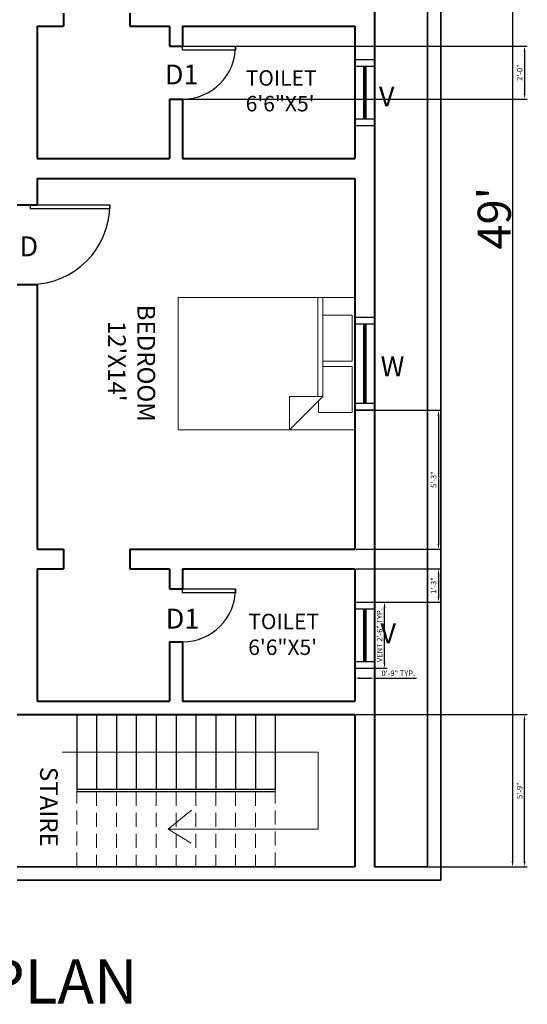
# Model space of a CAD drawing. Units: inches. Extents: x 6038 to 7543, y 3772 to 5131.
# Tile 6 of 14: x 6521 to 6751, y 4306 to 4753. Entities that reach past the tile are written whole.
import ezdxf

# ---------------------------------------------------------------- set-up
doc = ezdxf.new("R2010")
doc.units = ezdxf.units.IN
doc.linetypes.add('DASHED2', pattern=[9.525, 6.35, -3.175])
for name, color, linetype, lineweight in [('A-ANNO-DIMS', 4, 'Continuous', 18), ('A-ANNO-SYMB', 3, 'Continuous', 18), ('A-ANNO-TEXT', 7, 'Continuous', 18), ('A-ANNO-TITL', 3, 'Continuous', 30), ('A-AREA-IDEN', 2, 'Continuous', 18), ('A-DOOR', 3, 'Continuous', 25), ('A-FLOR-STRS', 7, 'Continuous', 25), ('A-FLOR-STRS-HIDN', 7, 'DASHED2', 18), ('A-FURN', 8, 'Continuous', 18), ('A-WALL', 7, 'Continuous', 40)]:
    doc.layers.add(name, color=color, linetype=linetype, lineweight=lineweight)
doc.layers.add('A-GLAZ', color=30, linetype='Continuous', lineweight=25, true_color=0xf26722)
doc.layers.add('C-PROP-WALL', color=251, linetype='Continuous', lineweight=35, true_color=0x636466)
doc.styles.get("Standard").update_dxf_attribs({"font": 'arial.ttf'})
doc.dimstyles.new('ISO-25', dxfattribs={"dimtxt": 2.5, "dimasz": 2.5, "dimexe": 1.25, "dimexo": 0.625, "dimtad": 1, "dimdec": 0, "dimlunit": 3, "dimtxsty": 'Standard', "dimcen": 2.5, "dimadec": 0, "dimazin": 0, "dimtfac": 1, "dimtdec": 0, "dimtmove": 0, "dimatfit": 3, "dimfxl": 1, "dimarcsym": 0})

# ---------------------------------------------------------------- blocks, each defined once
blk = doc.blocks.new('Bed - Queen')
for p, q in [((0, -80.00003), (0, 0)), ((0, 0), (59.99999, 0)), ((59.99999, 0), (59.99999, -80.00003)), ((7.99999, -1.2), (28.79998, -1.2)), ((7.99999, -14.4), (7.99999, -1.2)), ((28.79998, -1.2), (28.79998, -14.4)), ((31.19999, -1.2), (51.99999, -1.2)), ((31.19999, -14.4), (31.19999, -1.2)), ((51.99999, -1.2), (51.99999, -16.4)), ((0, -14.4), (44.8, -14.4)), ((44.8, -16.8), (0, -16.8)), ((59.99999, -29.6), (44.8, -14.4)), ((44.8, -14.4), (44.8, -29.6)), ((51.99999, -16.4), (46.79936, -16.4)), ((44.8, -29.6), (59.99999, -29.6)), ((59.99999, -80.00003), (0, -80.00003))]:
    blk.add_line(p, q)
blk = doc.blocks.new('*U9')
for p, q in [((0, 0), (0, -6)), ((36, 0), (36, -6))]:
    blk.add_line(p, q)
blk.add_lwpolyline([(0, 0), (0, 36), (1.75, 36), (1.75, 0)], close=True)
blk.add_arc((0, 0), 36, 0, 90)
blk = doc.blocks.new('*U8')
for p, q in [((0, 0), (0, -6)), ((24, 0), (24, -6))]:
    blk.add_line(p, q)
blk.add_lwpolyline([(0, 0), (0, 24), (1.75, 24), (1.75, 0)], close=True)
blk.add_arc((0, 0), 24, 0, 90)
blk = doc.blocks.new('*D14')
at = {"layer": 'A-ANNO-DIMS', "color": 0, "lineweight": -2, "transparency": 16777216}
for p, q in [((6682.04, 4956.62), (6745.18, 4956.62)), ((6743.93, 4954.12), (6743.93, 4371.12)), ((6682.04, 4368.62), (6745.18, 4368.62))]:
    blk.add_line(p, q, dxfattribs=at)
at = {"layer": 'A-ANNO-DIMS', "color": 0, "transparency": 16777216}
for points in [[(6743.51, 4954.12), (6744.35, 4954.12), (6743.93, 4956.62)], [(6743.51, 4371.12), (6744.35, 4371.12), (6743.93, 4368.62)]]:
    blk.add_solid(points, dxfattribs=at)
at = {"layer": 'Defpoints', "color": 0, "transparency": 16777216}
for p in [(6681.42, 4956.62), (6681.42, 4368.62), (6743.93, 4368.62)]:
    blk.add_point(p, dxfattribs=at)
at = {"layer": 'A-ANNO-DIMS', "color": 0, "transparency": 16777216, "insert": (6735.65, 4662.62), "char_height": 2.5, "attachment_point": 5, "rotation": 90}
blk.add_mtext("{\\H6x;49'}", dxfattribs=at)
blk = doc.blocks.new('WIN-36-PLAN')
for p, q in [((9, 42), (0, 42)), ((9, 39), (0, 39)), ((4, 39), (4, 3)), ((4.5, 39), (4.5, 3)), ((5, 39), (5, 3)), ((9, 3), (0, 3)), ((9, 0), (0, 0))]:
    blk.add_line(p, q)
blk = doc.blocks.new('VENT-24-PLAN')
for p, q in [((0, 30), (9, 30)), ((0, 27), (9, 27)), ((4, 27), (4, 3)), ((4.5, 27), (4.5, 3)), ((5, 27), (5, 3)), ((0, 3), (9, 3)), ((0, 0), (9, 0))]:
    blk.add_line(p, q)
blk = doc.blocks.new('*D34')
at = {"layer": 'A-ANNO-DIMS', "color": 0, "lineweight": -2, "transparency": 16777216}
for p, q in [((6682.04, 4488.62), (6687.17, 4488.62)), ((6685.92, 4461.12), (6685.92, 4486.12)), ((6682.04, 4458.62), (6687.17, 4458.62))]:
    blk.add_line(p, q, dxfattribs=at)
at = {"layer": 'A-ANNO-DIMS', "color": 0, "transparency": 16777216}
for points in [[(6685.5, 4486.12), (6686.33, 4486.12), (6685.92, 4488.62)], [(6685.5, 4461.12), (6686.33, 4461.12), (6685.92, 4458.62)]]:
    blk.add_solid(points, dxfattribs=at)
at = {"layer": 'Defpoints', "color": 0, "transparency": 16777216}
for p in [(6681.42, 4488.62), (6685.92, 4488.62), (6681.42, 4458.62)]:
    blk.add_point(p, dxfattribs=at)
at = {"layer": 'A-ANNO-DIMS', "color": 0, "transparency": 16777216, "insert": (6684.02, 4473.62), "char_height": 2.5, "attachment_point": 5, "rotation": 90}
blk.add_mtext('VENT 2\'-6" TYP.', dxfattribs=at)
blk = doc.blocks.new('*D35')
at = {"layer": 'A-ANNO-DIMS', "color": 0, "lineweight": -2, "transparency": 16777216}
for p, q in [((6672.42, 4457.99), (6672.42, 4452.87)), ((6681.42, 4457.99), (6681.42, 4452.87)), ((6674.92, 4454.12), (6678.92, 4454.12)), ((6681.42, 4454.12), (6700.41, 4454.12))]:
    blk.add_line(p, q, dxfattribs=at)
at = {"layer": 'A-ANNO-DIMS', "color": 0, "transparency": 16777216}
for points in [[(6674.92, 4454.54), (6674.92, 4453.7), (6672.42, 4454.12)], [(6678.92, 4454.54), (6678.92, 4453.7), (6681.42, 4454.12)]]:
    blk.add_solid(points, dxfattribs=at)
at = {"layer": 'Defpoints', "color": 0, "transparency": 16777216}
for p in [(6672.42, 4458.62), (6681.42, 4458.62), (6681.42, 4454.12)]:
    blk.add_point(p, dxfattribs=at)
at = {"layer": 'A-ANNO-DIMS', "color": 0, "transparency": 16777216, "insert": (6692.16, 4456.02), "char_height": 2.5, "attachment_point": 5}
blk.add_mtext('0\'-9" TYP.', dxfattribs=at)
blk = doc.blocks.new('*D56')
at = {"layer": 'A-ANNO-DIMS', "color": 0, "lineweight": -2, "transparency": 16777216}
for p, q in [((6673.04, 4437.62), (6750.62, 4437.62)), ((6749.37, 4371.12), (6749.37, 4435.12)), ((6682.04, 4368.62), (6750.62, 4368.62))]:
    blk.add_line(p, q, dxfattribs=at)
at = {"layer": 'A-ANNO-DIMS', "color": 0, "transparency": 16777216}
for points in [[(6748.95, 4435.12), (6749.78, 4435.12), (6749.37, 4437.62)], [(6748.95, 4371.12), (6749.78, 4371.12), (6749.37, 4368.62)]]:
    blk.add_solid(points, dxfattribs=at)
at = {"layer": 'Defpoints', "color": 0, "transparency": 16777216}
for p in [(6672.42, 4437.62), (6749.37, 4437.62), (6681.42, 4368.62)]:
    blk.add_point(p, dxfattribs=at)
at = {"layer": 'A-ANNO-DIMS', "color": 0, "transparency": 16777216, "insert": (6747.47, 4403.12), "char_height": 2.5, "attachment_point": 5, "rotation": 90}
blk.add_mtext('5\'-9"', dxfattribs=at)
blk = doc.blocks.new('*D59')
at = {"layer": 'A-ANNO-DIMS', "color": 0, "lineweight": -2, "transparency": 16777216}
for p, q in [((6589.04, 4740.62), (6750.62, 4740.62)), ((6749.37, 4738.12), (6749.37, 4719.12)), ((6589.04, 4716.62), (6750.62, 4716.62))]:
    blk.add_line(p, q, dxfattribs=at)
at = {"layer": 'A-ANNO-DIMS', "color": 0, "transparency": 16777216}
for points in [[(6748.95, 4738.12), (6749.78, 4738.12), (6749.37, 4740.62)], [(6748.95, 4719.12), (6749.78, 4719.12), (6749.37, 4716.62)]]:
    blk.add_solid(points, dxfattribs=at)
at = {"layer": 'Defpoints', "color": 0, "transparency": 16777216}
for p in [(6588.42, 4740.62), (6588.42, 4716.62), (6749.37, 4716.62)]:
    blk.add_point(p, dxfattribs=at)
at = {"layer": 'A-ANNO-DIMS', "color": 0, "transparency": 16777216, "insert": (6747.47, 4728.62), "char_height": 2.5, "attachment_point": 5, "rotation": 90}
blk.add_mtext('2\'-0"', dxfattribs=at)
blk = doc.blocks.new('*D61')
at = {"layer": 'A-ANNO-DIMS', "color": 0, "lineweight": -2, "transparency": 16777216}
for p, q in [((6673.04, 4575.62), (6711.62, 4575.62)), ((6710.37, 4573.12), (6710.37, 4515.12)), ((6673.04, 4512.62), (6711.62, 4512.62))]:
    blk.add_line(p, q, dxfattribs=at)
at = {"layer": 'A-ANNO-DIMS', "color": 0, "transparency": 16777216}
for points in [[(6709.95, 4573.12), (6710.78, 4573.12), (6710.37, 4575.62)], [(6709.95, 4515.12), (6710.78, 4515.12), (6710.37, 4512.62)]]:
    blk.add_solid(points, dxfattribs=at)
at = {"layer": 'Defpoints', "color": 0, "transparency": 16777216}
for p in [(6672.42, 4575.62), (6672.42, 4512.62), (6710.37, 4512.62)]:
    blk.add_point(p, dxfattribs=at)
at = {"layer": 'A-ANNO-DIMS', "color": 0, "transparency": 16777216, "insert": (6708.46, 4544.12), "char_height": 2.5, "attachment_point": 5, "rotation": 90}
blk.add_mtext('5\'-3"', dxfattribs=at)
blk = doc.blocks.new('*D65')
at = {"layer": 'A-ANNO-DIMS', "color": 0, "lineweight": -2, "transparency": 16777216}
for p, q in [((6673.04, 4503.62), (6711.62, 4503.62)), ((6710.37, 4501.12), (6710.37, 4491.12)), ((6673.04, 4488.62), (6711.62, 4488.62))]:
    blk.add_line(p, q, dxfattribs=at)
at = {"layer": 'A-ANNO-DIMS', "color": 0, "transparency": 16777216}
for points in [[(6709.95, 4501.12), (6710.78, 4501.12), (6710.37, 4503.62)], [(6709.95, 4491.12), (6710.78, 4491.12), (6710.37, 4488.62)]]:
    blk.add_solid(points, dxfattribs=at)
at = {"layer": 'Defpoints', "color": 0, "transparency": 16777216}
for p in [(6672.42, 4503.62), (6672.42, 4488.62), (6710.37, 4488.62)]:
    blk.add_point(p, dxfattribs=at)
at = {"layer": 'A-ANNO-DIMS', "color": 0, "transparency": 16777216, "insert": (6708.46, 4496.12), "char_height": 2.5, "attachment_point": 5, "rotation": 90}
blk.add_mtext('1\'-3"', dxfattribs=at)

msp = doc.modelspace()

# ---------------------------------------------------------------- linework, layer by layer
at = {"layer": 'A-ANNO-SYMB'}
for p, q in [((6539.88, 4420.62), (6655.84, 4420.62)), ((6655.84, 4420.62), (6655.84, 4385.62)), ((6587.85, 4385.62), (6598.47, 4394.32)), ((6655.84, 4385.62), (6587.85, 4385.62)), ((6587.85, 4385.62), (6598.27, 4379.35))]:
    msp.add_line(p, q, dxfattribs=at)
at = {"layer": 'A-FLOR-STRS'}
for p, q in [((6546.42, 4437.62), (6546.42, 4403.62)), ((6555.42, 4437.62), (6555.42, 4403.62)), ((6564.42, 4437.62), (6564.42, 4403.62)), ((6573.42, 4437.62), (6573.42, 4403.62)), ((6582.42, 4437.62), (6582.42, 4403.62)), ((6591.42, 4437.62), (6591.42, 4403.62)), ((6600.42, 4437.62), (6600.42, 4403.62)), ((6609.42, 4437.62), (6609.42, 4403.62)), ((6618.42, 4437.62), (6618.42, 4403.62)), ((6627.42, 4437.62), (6627.42, 4403.62)), ((6636.42, 4437.62), (6636.42, 4403.62)), ((6636.42, 4403.62), (6546.42, 4403.62)), ((6636.42, 4402.62), (6546.42, 4402.62))]:
    msp.add_line(p, q, dxfattribs=at)
at = {"layer": 'A-FLOR-STRS-HIDN'}
for p, q in [((6546.42, 4403.62), (6546.42, 4368.62)), ((6555.42, 4402.62), (6555.42, 4368.62)), ((6564.42, 4402.62), (6564.42, 4368.62)), ((6573.42, 4402.62), (6573.42, 4368.62)), ((6582.42, 4402.62), (6582.42, 4368.62)), ((6591.42, 4402.62), (6591.42, 4368.62)), ((6600.42, 4402.62), (6600.42, 4368.62)), ((6609.42, 4402.62), (6609.42, 4368.62)), ((6618.42, 4402.62), (6618.42, 4368.62)), ((6627.42, 4402.62), (6627.42, 4368.62)), ((6636.42, 4403.62), (6636.42, 4368.62))]:
    msp.add_line(p, q, dxfattribs=at)
at = {"layer": 'A-WALL'}
for p, q in [((6681.42, 4956.62), (6681.42, 4368.62)), ((6540.42, 4755.62), (6540.42, 4749.62)), ((6570.42, 4755.62), (6570.42, 4749.62)), ((6528.42, 4749.62), (6540.42, 4749.62)), ((6528.42, 4749.62), (6528.42, 4689.62)), ((6570.42, 4749.62), (6588.42, 4749.62)), ((6588.42, 4749.62), (6588.42, 4740.62)), ((6594.42, 4749.62), (6594.42, 4740.62)), ((6594.42, 4749.62), (6672.42, 4749.62)), ((6672.42, 4749.62), (6672.42, 4689.62)), ((6588.42, 4740.62), (6594.42, 4740.62)), ((6588.42, 4716.62), (6594.42, 4716.62)), ((6588.42, 4716.62), (6588.42, 4689.62)), ((6594.42, 4716.62), (6594.42, 4689.62)), ((6528.42, 4689.62), (6588.42, 4689.62)), ((6594.42, 4689.62), (6672.42, 4689.62)), ((6528.42, 4680.62), (6672.42, 4680.62)), ((6528.42, 4680.62), (6528.42, 4668.62)), ((6672.42, 4680.62), (6672.42, 4512.62)), ((6519.42, 4668.62), (6528.42, 4668.62)), ((6519.42, 4632.62), (6528.42, 4632.62)), ((6528.42, 4632.62), (6528.42, 4512.62)), ((6528.42, 4512.62), (6540.42, 4512.62)), ((6540.42, 4512.62), (6540.42, 4503.62)), ((6570.42, 4512.62), (6570.42, 4503.62)), ((6570.42, 4512.62), (6672.42, 4512.62)), ((6528.42, 4503.62), (6540.42, 4503.62)), ((6528.42, 4503.62), (6528.42, 4443.62)), ((6570.42, 4503.62), (6588.42, 4503.62)), ((6588.42, 4503.62), (6588.42, 4494.62)), ((6594.42, 4503.62), (6594.42, 4494.62)), ((6594.42, 4503.62), (6672.42, 4503.62)), ((6672.42, 4503.62), (6672.42, 4443.62)), ((6588.42, 4494.62), (6594.42, 4494.62)), ((6588.42, 4470.62), (6594.42, 4470.62)), ((6588.42, 4470.62), (6588.42, 4443.62)), ((6594.42, 4470.62), (6594.42, 4443.62)), ((6528.42, 4443.62), (6588.42, 4443.62)), ((6594.42, 4443.62), (6672.42, 4443.62)), ((6519.42, 4437.62), (6672.42, 4437.62)), ((6672.42, 4437.62), (6672.42, 4368.62))]:
    msp.add_line(p, q, dxfattribs=at)
at = {"layer": 'C-PROP-WALL'}
for p, q in [((6711.42, 4986.62), (6711.42, 4362.62)), ((6705.42, 4980.62), (6705.42, 4368.62)), ((6672.42, 4368.62), (6519.42, 4368.62)), ((6705.42, 4368.62), (6681.42, 4368.62)), ((6711.42, 4362.62), (6519.42, 4362.62))]:
    msp.add_line(p, q, dxfattribs=at)

# ---------------------------------------------------------------- block references
at = {"layer": 'A-DOOR', "rotation": 270}
for name, p in [('*U8', (6594.42, 4740.62)), ('*U9', (6525.42, 4668.62)), ('*U8', (6594.42, 4494.62))]:
    msp.add_blockref(name, p, dxfattribs=at)
at = {"layer": 'A-FURN', "rotation": 270}
msp.add_blockref('Bed - Queen', (6672.42, 4626.62), dxfattribs=at)
at = {"layer": 'A-GLAZ'}
for name, p in [('VENT-24-PLAN', (6672.42, 4704.62)), ('WIN-36-PLAN', (6672.42, 4575.62)), ('VENT-24-PLAN', (6672.42, 4458.62))]:
    msp.add_blockref(name, p, dxfattribs=at)

# ---------------------------------------------------------------- texts
at = {"layer": 'A-ANNO-TEXT', "char_height": 9, "attachment_point": 1}
for s, insert in [('D1', (6586.35, 4732.27)), ('V', (6683.37, 4722.33)), ('D', (6520.5, 4654.37)), ('W', (6684.15, 4599.94)), ('D1', (6586.73, 4485.6)), ('V', (6684.05, 4478.96))]:
    msp.add_mtext_dynamic_manual_height_columns(s, width=212.1416, gutter_width=12.5, heights=[0], dxfattribs=dict(at, insert=insert))
at = {"layer": 'A-ANNO-TITL', "insert": (6411.79, 4326.63), "char_height": 20, "attachment_point": 1}
msp.add_mtext_dynamic_manual_height_columns('FLOOR PLAN', width=549.9641, gutter_width=12.5, heights=[0], dxfattribs=at)
at = {"layer": 'A-AREA-IDEN', "char_height": 7, "attachment_point": 1}
for insert in [(6622.98, 4729.72), (6624.14, 4483.31)]:
    msp.add_mtext_dynamic_manual_height_columns('TOILET\\P6\'6"X5\'', width=333.3072, gutter_width=12.5, heights=[0], dxfattribs=dict(at, insert=insert))
at = {"layer": 'A-AREA-IDEN', "char_height": 8, "attachment_point": 1, "rotation": 270}
for s, width, insert in [("BEDROOM\\P   12'X14'", 589.9095, (6581.96, 4623.42)), ('STAIRE', 620.4895, (6537.82, 4413.92))]:
    msp.add_mtext_dynamic_manual_height_columns(s, width=width, gutter_width=12.5, heights=[0], dxfattribs=dict(at, insert=insert))

# ---------------------------------------------------------------- dimensions: what is measured, and where the dimension line sits
at = {"layer": 'A-ANNO-DIMS'}
for base, p1, p2, text, override, picture, middle in [((6743.93, 4368.62), (6681.42, 4956.62), (6681.42, 4368.62), '{\\H6x;<>}', {"dimclrd": 0, "dimclre": 0, "dimclrt": 0}, '*D14', (6735.65, 4662.62)), ((6685.92, 4488.62), (6681.42, 4458.62), (6681.42, 4488.62), 'VENT <> TYP.', {"dimdec": 1, "dimlfac": 1, "dimrnd": 0, "dimzin": 1, "dimdsep": 46, "dimlunit": 4, "dimfrac": 2}, '*D34', (6684.02, 4473.62))]:
    dim = msp.add_linear_dim(base=base, p1=p1, p2=p2, angle=90, text=text, dimstyle='ISO-25', override=override, dxfattribs=at)
    dim.commit()
    dim.dimension.update_dxf_attribs({"geometry": picture, "text_midpoint": middle})
for base, p1, p2, angle, picture, middle in [((6749.37, 4716.62), (6588.42, 4740.62), (6588.42, 4716.62), 90, '*D59', (6747.47, 4728.62)), ((6710.37, 4512.62), (6672.42, 4575.62), (6672.42, 4512.62), 270, '*D61', (6708.46, 4544.12)), ((6710.37, 4488.62), (6672.42, 4503.62), (6672.42, 4488.62), 270, '*D65', (6708.46, 4496.12)), ((6749.37, 4437.62), (6681.42, 4368.62), (6672.42, 4437.62), 90, '*D56', (6747.47, 4403.12))]:
    dim = msp.add_linear_dim(base=base, p1=p1, p2=p2, angle=angle, dimstyle='ISO-25', override={"dimdec": 1, "dimlfac": 1, "dimrnd": 0, "dimzin": 1, "dimdsep": 46, "dimlunit": 4, "dimfrac": 2}, dxfattribs=at)
    dim.commit()
    dim.dimension.update_dxf_attribs({"geometry": picture, "text_midpoint": middle})
dim = msp.add_linear_dim(base=(6681.42, 4454.12), p1=(6672.42, 4458.62), p2=(6681.42, 4458.62), text='<> TYP.', dimstyle='ISO-25', override={"dimdec": 1, "dimlfac": 1, "dimrnd": 0, "dimzin": 1, "dimdsep": 46, "dimlunit": 4, "dimfrac": 2}, dxfattribs=at)
dim.commit()
dim.dimension.update_dxf_attribs({"geometry": '*D35', "text_midpoint": (6692.16, 4456.02)})

doc.saveas('drawing.dxf')
